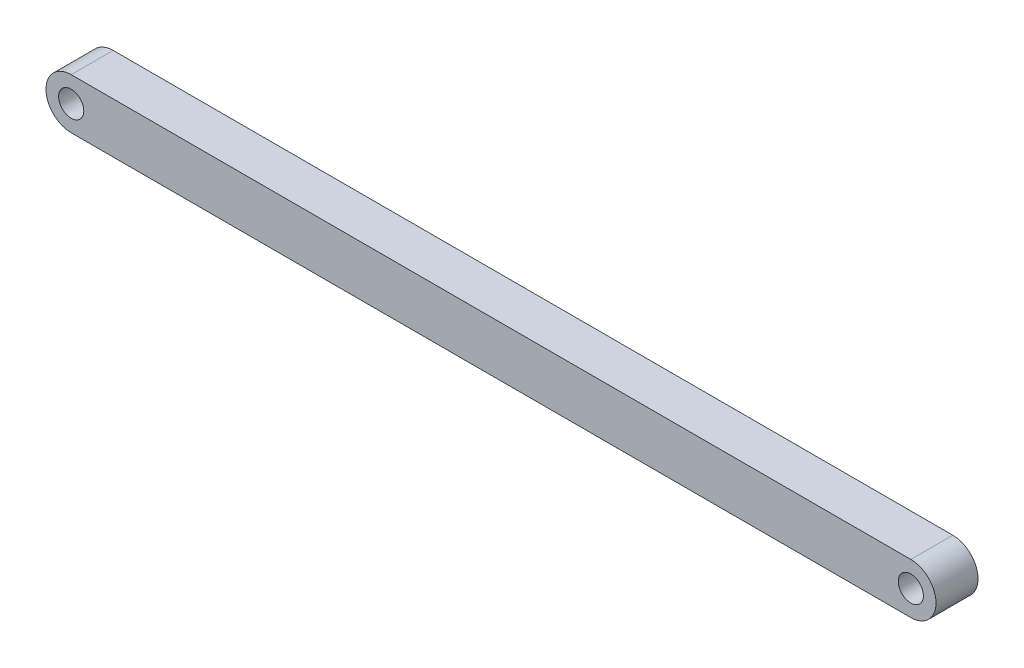
SolidWorks part; units mm, degrees
material "Plain Carbon Steel"
ref_plane "Front Plane" through (0, 0, 0) normal (0, 0, 1) x (1, 0, 0)
ref_plane "Top Plane" through (0, 0, 0) normal (0, 1, 0) x (1, 0, 0)
ref_plane "Right Plane" through (0, 0, 0) normal (1, 0, 0) x (0, 0, -1)
sketch "Link Profile Sketch" plane through (0, 0, 0) normal (0, 0, 1) x (1, 0, 0)
  line L0 (-50, 0) -> (50, 0) construction
  line L1 (-50, 3) -> (50, 3)
  line L2 (-50, -3) -> (50, -3)
  arc A0 (-50, 3) -> (-50, -3) centre (-50, 0) ccw
  arc A1 (50, -3) -> (50, 3) centre (50, 0) ccw
  circle A2 centre (-50, 0) radius 1.5
  circle A3 centre (50, 0) radius 1.5
  point P2 (0, 0)
  dimension "D2" = 3
  dimension "D3" = 3
  dimension "D4" = 3
  dimension "D1" = 100
extrude "Link Bar 100 Ctrs 2xØ3" add sketch "Link Profile Sketch" along normal blind 5
